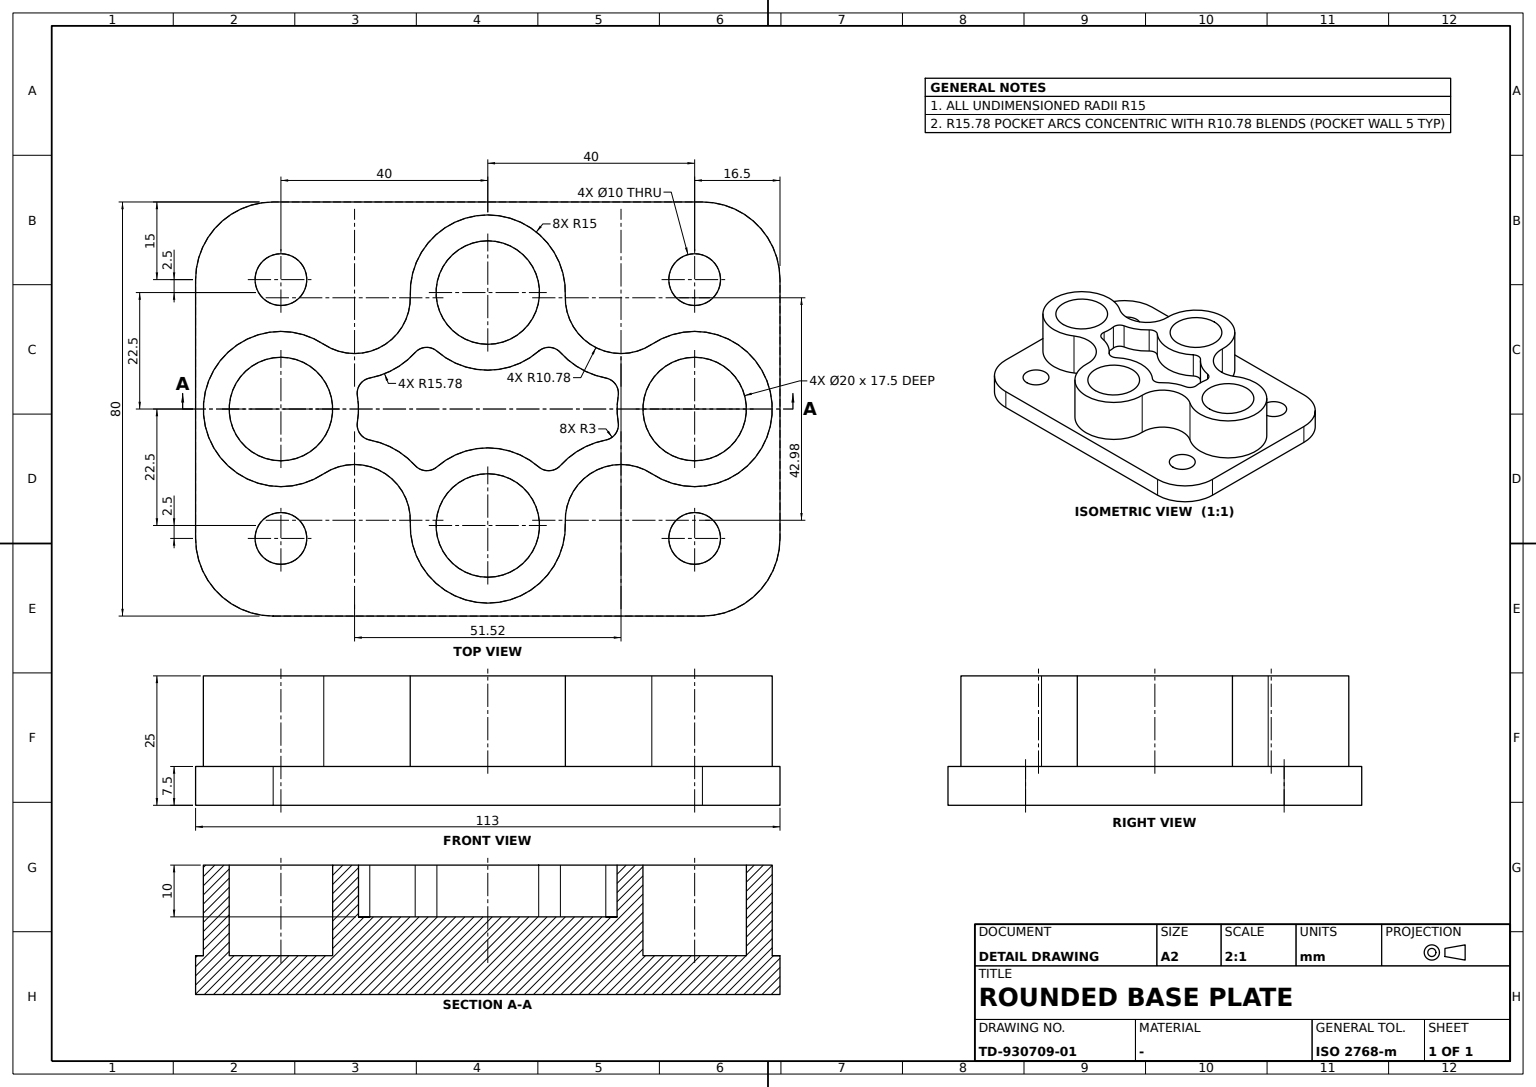
CATIA V5 part; units mm, degrees
sketch "Sketch1" plane through (0, 0, 0) normal (0, 0, 1) x (1, 0, 0)
  line L0 (40, 41.5) -> (40, -41.5)
  line L1 (25, -56.5) -> (-25, -56.5)
  line L2 (-40, -41.5) -> (-40, 41.5)
  line L3 (-25, 56.5) -> (25, 56.5)
  point P0 (40, 56.5)
  point P1 (40, -56.5)
  point P2 (-40, -56.5)
  arc A0 (25, 56.5) -> (40, 41.5) centre (25, 41.5) cw
  arc A1 (-25, 56.5) -> (-40, 41.5) centre (-25, 41.5) ccw
  arc A2 (-25, -56.5) -> (-40, -41.5) centre (-25, -41.5) cw
  arc A3 (25, -56.5) -> (40, -41.5) centre (25, -41.5) ccw
  dimension "distance P0 P1" = 113
  dimension "radius A0" = 15
  dimension "radius A1" = 15
  dimension "distance P1 P2" = 80
  dimension "radius A2" = 15
  dimension "radius A3" = 15
  constraint vertical L0 y-axis
  constraint vertical L2 y-axis
  constraint horizontal L1 x-axis
  constraint horizontal L3 x-axis
  constraint equidistance L0 L2 origin
  constraint equidistance L1 L3 origin
  constraint coincidence L3 P0
  constraint coincidence L0 P0
  constraint coincidence L1 P2
  constraint coincidence L2 P2
  constraint coincidence L1 P1
  constraint coincidence L0 P1
  constraint tangency A0 L3
  constraint tangency A0 L0
  constraint tangency A1 L3
  constraint tangency A1 L2
  constraint tangency A2 L1
  constraint tangency A2 L2
  constraint tangency A3 L1
  constraint tangency A3 L0
extrude "Pad1" add sketch "Sketch1" along normal blind 7.5
sketch "Sketch2" plane through (0, 0, 7.5) normal (0, 0, 1) x (1, 0, 0)
  circle A0 centre (-25, 40) radius 5
  point P0 (-25, 40)
  circle A1 centre (25, 40) radius 5
  point P1 (25, 40)
  circle A2 centre (-25, -40) radius 5
  circle A3 centre (25, -40) radius 5
  dimension "radius A0" = 5
  dimension "distance P0 x axis" = 40
  dimension "distance P0 y axis" = 25
  dimension "radius A1" = 5
  dimension "distance P1 y axis" = 25
  dimension "distance P1 x axis" = 40
  constraint symmetry A0 A2 x-axis
  constraint symmetry A1 A3 x-axis
extrude "Pocket1" cut sketch "Sketch2" against normal blind 7.5
sketch "Sketch3" plane through (0, 0, 7.5) normal (0, 0, 1) x (1, 0, 0)
  point P0 (22.5, 0)
  point P1 (-22.5, 0)
  point P2 (0, 40)
  arc A0 (-21.9133, 14.9885) -> (-21.9133, -14.9885) centre (-22.5, 0) ccw
  arc A1 (21.9133, 14.9885) -> (21.9133, -14.9885) centre (22.5, 0) cw
  arc A2 (12.5045, 31.7152) -> (-12.5045, 31.7152) centre (0, 40) ccw
  arc A3 (12.5045, -31.7152) -> (-12.5045, -31.7152) centre (0, -40) cw
  arc A4 (12.5045, 31.7152) -> (21.9133, 14.9885) centre (21.4915, 25.7609) ccw
  point P3 (21.4915, 25.7609)
  point P4 (-21.4915, 25.7609)
  arc A5 (-12.5045, 31.7152) -> (-21.9133, 14.9885) centre (-21.4915, 25.7609) cw
  arc A6 (-12.5045, -31.7152) -> (-21.9133, -14.9885) centre (-21.4915, -25.7609) ccw
  arc A7 (12.5045, -31.7152) -> (21.9133, -14.9885) centre (21.4915, -25.7609) cw
  dimension "distance P0 y axis" = 22.5
  dimension "distance P2 x axis" = 40
  dimension "radius A0" = 15
  dimension "radius A2" = 15
  dimension "distance P3 x axis" = 25.7609
  dimension "distance P4 y axis" = 21.4915
  dimension "distance P1 y axis" = 22.5
  constraint coincidence P0 x-axis
  constraint coincidence P2 y-axis
  constraint symmetry A0 A1 y-axis
  constraint symmetry A2 A3 x-axis
  constraint symmetry A4 A5 y-axis
  constraint symmetry A5 A6 x-axis
  constraint symmetry A6 A7 y-axis
  constraint tangency A4 A2
  constraint tangency A4 A1
extrude "Pad2" add sketch "Sketch3" along normal blind 17.5
sketch "Sketch4" plane through (0, 0, 25) normal (0, 0, 1) x (1, 0, 0)
  circle A0 centre (0, 40) radius 10
  point P0 (0, 40)
  arc A1 (12.5045, 31.7152) -> (-12.5045, 31.7152) centre (0, 40) ccw construction
  circle A2 centre (0, -40) radius 10
  circle A3 centre (22.5, 0) radius 10
  point P1 (22.5, 0)
  arc A4 (21.9133, -14.9885) -> (21.9133, 14.9885) centre (22.5, 0) ccw construction
  circle A5 centre (-22.5, 0) radius 10
  dimension "radius A0" = 10
  dimension "radius A3" = 10
  constraint coincidence P0 y-axis
  constraint coincidence P1 x-axis
  constraint concentricity A0 A1
  constraint concentricity A3 A4
  constraint symmetry A0 A2 x-axis
  constraint symmetry A3 A5 y-axis
extrude "Pocket2" cut sketch "Sketch4" against normal blind 17.5
sketch "Sketch5" plane through (0, 0, 25) normal (0, 0, 1) x (1, 0, 0)
  arc A0 (-2.5337, 25.2155) -> (2.5337, 25.2155) centre (0, 40) ccw
  point P0 (0, 40)
  circle A1 centre (0, 40) radius 10 construction
  arc A2 (-2.5337, -25.2155) -> (2.5337, -25.2155) centre (0, -40) cw
  arc A3 (-11.1809, -9.8427) -> (-11.1809, 9.8427) centre (-22.5, 0) ccw
  point P1 (-22.5, 0)
  circle A4 centre (-22.5, 0) radius 10 construction
  arc A5 (11.1809, -9.8427) -> (11.1809, 9.8427) centre (22.5, 0) cw
  arc A6 (-22.1088, 9.9923) -> (-8.3363, 34.4768) centre (-21.4915, 25.7609) ccw construction
  arc A7 (-10.9257, 14.0395) -> (-5.9878, 22.8181) centre (-21.4915, 25.7609) ccw
  point P2 (-22.1088, 9.9923)
  point P3 (-8.3363, 34.4768)
  arc A8 (10.9257, 14.0395) -> (5.9878, 22.8181) centre (21.4915, 25.7609) cw
  point P4 (22.1088, 9.9923)
  point P5 (8.3363, 34.4768)
  point P6 (8.3363, -34.4768)
  point P7 (22.1088, -9.9923)
  arc A9 (10.9257, -14.0395) -> (5.9878, -22.8181) centre (21.4915, -25.7609) ccw
  arc A10 (-10.9257, -14.0395) -> (-5.9878, -22.8181) centre (-21.4915, -25.7609) cw
  point P8 (-5.7153, 26.1315)
  point P9 (-13.6159, 12.086)
  arc A11 (-5.9878, 22.8181) -> (-2.5337, 25.2155) centre (-3.0404, 22.2586) cw
  arc A12 (2.5337, 25.2155) -> (5.9878, 22.8181) centre (3.0404, 22.2586) cw
  arc A13 (10.9257, 14.0395) -> (11.1809, 9.8427) centre (8.9171, 11.8112) cw
  arc A14 (11.1809, -9.8427) -> (10.9257, -14.0395) centre (8.9171, -11.8112) cw
  arc A15 (2.5337, -25.2155) -> (5.9878, -22.8181) centre (3.0404, -22.2586) ccw
  arc A16 (-2.5337, -25.2155) -> (-5.9878, -22.8181) centre (-3.0404, -22.2586) cw
  arc A17 (-10.9257, -14.0395) -> (-11.1809, -9.8427) centre (-8.9171, -11.8112) cw
  arc A18 (-10.9257, 14.0395) -> (-11.1809, 9.8427) centre (-8.9171, 11.8112) ccw
  dimension "radius A0" = 15
  dimension "radius A3" = 15
  dimension "radius A11" = 3
  dimension "radius A12" = 3
  dimension "radius A13" = 3
  dimension "radius A14" = 3
  dimension "radius A15" = 3
  dimension "radius A16" = 3
  dimension "radius A17" = 3
  dimension "radius A18" = 3
  constraint coincidence P0 y-axis
  constraint coincidence P1 x-axis
  constraint coincidence A6 P8
  constraint coincidence A6 P9
  constraint coincidence A0 P8
  constraint coincidence A3 P9
  constraint concentricity A0 A1
  constraint concentricity A3 A4
  constraint symmetry A0 A2 x-axis
  constraint symmetry A3 A5 y-axis
  constraint symmetry A6 A8 y-axis
  constraint symmetry P2 P4 y-axis
  constraint symmetry P3 P5 y-axis
  constraint symmetry P5 P6 x-axis
  constraint symmetry P4 P7 x-axis
  constraint symmetry A8 A9 x-axis
  constraint symmetry A9 A10 y-axis
  constraint tangency A11 A6
  constraint tangency A11 A0
  constraint tangency A12 A0
  constraint tangency A12 A8
  constraint tangency A13 A8
  constraint tangency A13 A5
  constraint tangency A14 A5
  constraint tangency A14 A9
  constraint tangency A15 A2
  constraint tangency A15 A9
  constraint tangency A16 A2
  constraint tangency A16 A10
  constraint tangency A17 A10
  constraint tangency A17 A3
  constraint tangency A18 A6
  constraint tangency A18 A3
extrude "Pocket3" cut sketch "Sketch5" against normal blind 10
